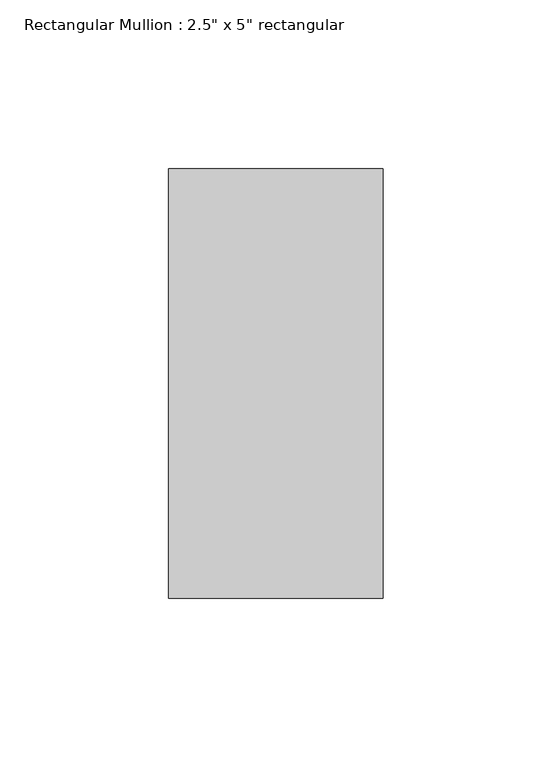
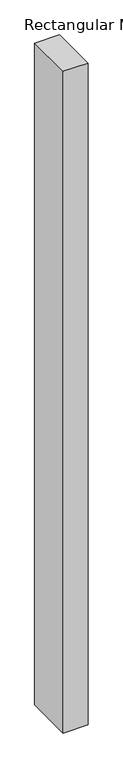
"""IFC4 building model written with IfcOpenShell, lengths in millimetres: member geometry."""

from ifc_helpers import new_model, si_unit, frame, origin, place, context, project, spatial, polyline, outline, extrude, source, transform, mapped, element, save


def member_3fd415ec(model_context):
    return source(origin(), model_context, "Body", "SweptSolid", [
        extrude(outline(polyline([(31.75, 63.5), (31.75, -63.5), (-31.75, -63.5), (-31.75, 63.5), (31.75, 63.5)])), frame((0.0, 0.0, -1796.4671151), z_axis=(0.0, 0.0, 1.0), x_axis=(1.0, 0.0, 0.0)), (0.0, 0.0, 1.0), 1796.4671151),
    ])


if __name__ == "__main__":
    model = new_model("IFC4")
    model_context = context("Model", 3, world=origin())
    ifc_project = project(units=[si_unit("LENGTHUNIT", "METRE", prefix="MILLI")], contexts=[model_context])
    site = spatial("IfcSite", under=ifc_project)
    building = spatial("IfcBuilding", under=site)
    placement = place(None, origin())
    member_shape = member_3fd415ec(model_context)
    element("IfcMember", 1, ObjectType="Rectangular Mullion : 2.5\" x 5\" rectangular", at=placement, inside=building, context=model_context, shape_type="MappedRepresentation", body=[
        mapped(member_shape, transform((0.0, 0.0, 0.0), x_axis=(1.0, 0.0, 0.0), y_axis=(0.0, 1.0, 0.0), z_axis=(0.0, 0.0, 1.0))),
    ])
    save(model, "model.ifc")

# Revit data of these elements
# Type "Rectangular Mullion : 2.5\" x 5\" rectangular"
#   built-in parameter 1007304 = 0.416667 (stored number, unit not read)
#   built-in parameter 1007301 = 0.104167 (stored number, unit not read)
#   built-in parameter 1007300 = 0.104167 (stored number, unit not read)
# Element 1 (IfcMember, "Rectangular Mullion : 2.5\" x 5\" rectangular")
#   Materials on its faces: "Aluminum"
# Materials
#   "Aluminum": class "Metal", colour RGB 247 247 247, transparency 0, Description = "Aluminum 6061", Cost = 0
